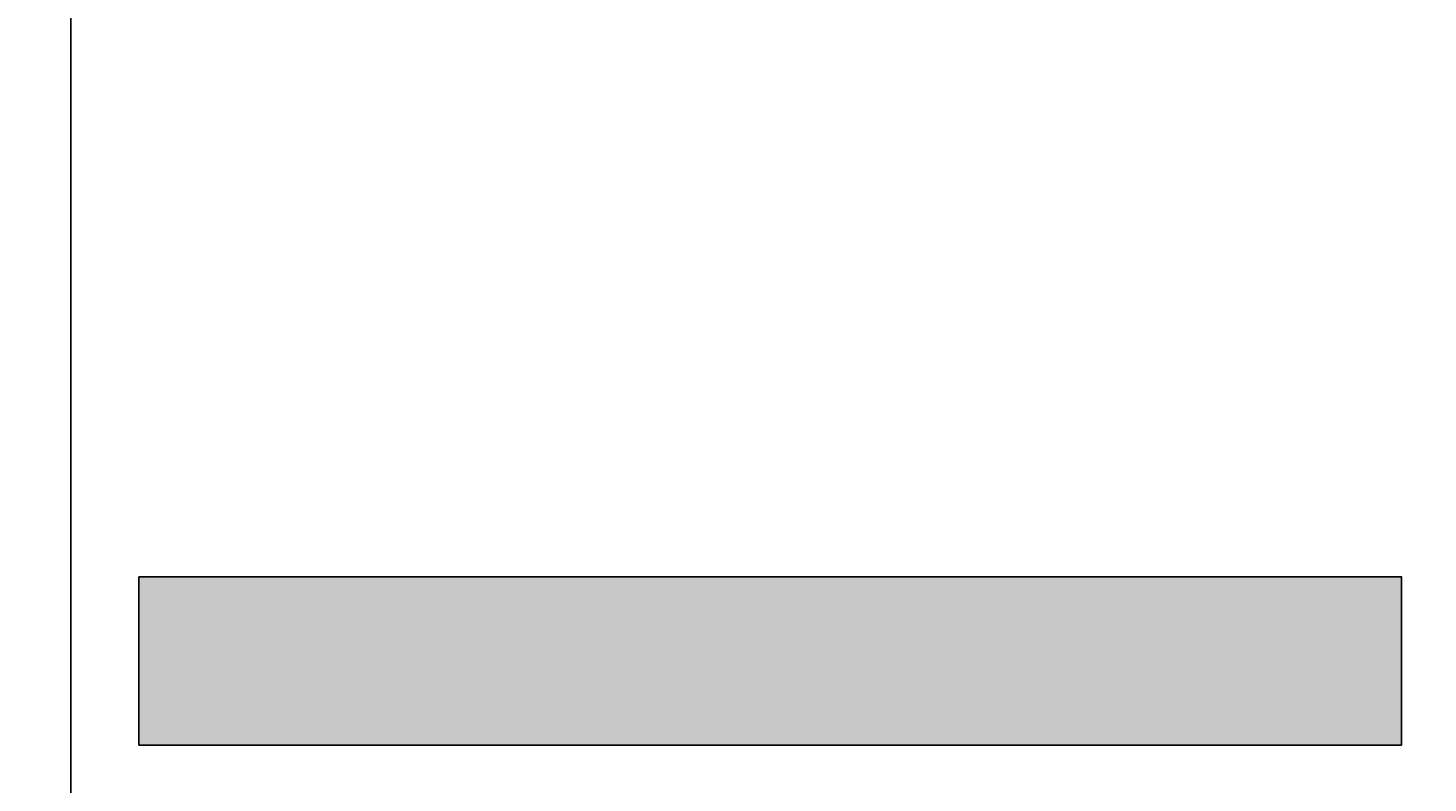
# Model space of a CAD drawing. Units: millimetres. Extents: x -11 to 280, y -4 to 208.
# Tile 3 of 55: x 28 to 61, y 36 to 54. Entities that reach past the tile are written whole.
import ezdxf

# ---------------------------------------------------------------- set-up
doc = ezdxf.new("R2010")
doc.units = ezdxf.units.MM
doc.layers.add('M-DIMS', color=2, linetype='Continuous', lineweight=18)
doc.layers.add('M-HYDR-SUCT', color=7, linetype='Continuous', lineweight=25)
doc.layers.add('M-HYDR-SUCT-PATT', color=221, linetype='Continuous', lineweight=13, true_color=0xff7fdf)
doc.styles.get("Standard").update_dxf_attribs({"font": 'arial.ttf'})
doc.dimstyles.get("Standard").update_dxf_attribs({"dimtxt": 0.18, "dimasz": 0.18, "dimexe": 0.18, "dimexo": 0.0625, "dimgap": 0.09, "dimtad": 0, "dimtih": 1, "dimtoh": 1, "dimdec": 4, "dimzin": 0, "dimdsep": 46, "dimtxsty": 'Standard', "dimcen": 0.09, "dimadec": 0, "dimazin": 0, "dimtfac": 1, "dimtdec": 4, "dimtofl": 0, "dimtmove": 0, "dimatfit": 3, "dimfxl": 1, "dimtolj": 1, "dimtzin": 0, "dimarcsym": 0})

# ---------------------------------------------------------------- blocks, each defined once
blk = doc.blocks.new('*D4')
at = {"layer": 'Defpoints', "color": 0, "transparency": 16777216}
for p in [(4.763, 84.426), (266.035, 51.733), (266.035, -3.415)]:
    blk.add_point(p, dxfattribs=at)
at = {"layer": 'M-DIMS', "color": 0, "lineweight": -2, "transparency": 16777216}
for p, q in [((4.763, 84.364), (4.763, -3.595)), ((266.035, 51.67), (266.035, -3.595)), ((4.943, -3.415), (134.934, -3.415)), ((265.855, -3.415), (135.864, -3.415))]:
    blk.add_line(p, q, dxfattribs=at)
at = {"layer": 'M-DIMS', "color": 0, "transparency": 16777216}
for points in [[(4.943, -3.385), (4.943, -3.445), (4.763, -3.415)], [(265.855, -3.385), (265.855, -3.445), (266.035, -3.415)]]:
    blk.add_solid(points, dxfattribs=at)
at = {"layer": 'M-DIMS', "color": 0, "transparency": 16777216, "insert": (135.399, -3.415), "char_height": 0.18, "attachment_point": 5}
blk.add_mtext('\\A1;261.27', dxfattribs=at)
blk = doc.blocks.new('*D5')
at = {"layer": 'Defpoints', "color": 0, "transparency": 16777216}
for p in [(24.759, 192.645), (-10.087, 11.435), (261.686, 11.435)]:
    blk.add_point(p, dxfattribs=at)
at = {"layer": 'M-DIMS', "color": 0, "lineweight": -2, "transparency": 16777216}
for p, q in [((24.696, 192.645), (-10.267, 192.645)), ((-10.087, 192.465), (-10.087, 102.222)), ((-10.087, 11.615), (-10.087, 101.858)), ((261.624, 11.435), (-10.267, 11.435))]:
    blk.add_line(p, q, dxfattribs=at)
at = {"layer": 'M-DIMS', "color": 0, "transparency": 16777216}
for points in [[(-10.117, 192.465), (-10.057, 192.465), (-10.087, 192.645)], [(-10.117, 11.615), (-10.057, 11.615), (-10.087, 11.435)]]:
    blk.add_solid(points, dxfattribs=at)
at = {"layer": 'M-DIMS', "color": 0, "transparency": 16777216, "insert": (-10.087, 102.04), "char_height": 0.18, "attachment_point": 5}
blk.add_mtext('\\A1;181.2', dxfattribs=at)
blk = doc.blocks.new('*D23')
at = {"layer": 'Defpoints', "color": 0, "transparency": 16777216}
for p in [(29.201, 153.977), (66.388, 153.977), (66.388, -3.415)]:
    blk.add_point(p, dxfattribs=at)
at = {"layer": 'M-DIMS', "color": 0, "lineweight": -2, "transparency": 16777216}
for p, q in [((29.201, 153.914), (29.201, -3.595)), ((66.388, 153.914), (66.388, -3.595)), ((29.381, -3.415), (47.331, -3.415)), ((66.208, -3.415), (48.258, -3.415))]:
    blk.add_line(p, q, dxfattribs=at)
at = {"layer": 'M-DIMS', "color": 0, "transparency": 16777216}
for points in [[(29.381, -3.385), (29.381, -3.445), (29.201, -3.415)], [(66.208, -3.385), (66.208, -3.445), (66.388, -3.415)]]:
    blk.add_solid(points, dxfattribs=at)
at = {"layer": 'M-DIMS', "color": 0, "transparency": 16777216, "insert": (47.795, -3.415), "char_height": 0.18, "attachment_point": 5}
blk.add_mtext('\\A1;37.186', dxfattribs=at)

msp = doc.modelspace()

# ---------------------------------------------------------------- hatches: boundary and pattern name
at = {"layer": 'M-HYDR-SUCT-PATT'}
h = msp.add_hatch(color=256, dxfattribs=at)
h.set_gradient(color1=(255, 127, 223), color2=(255, 127, 223), tint=1, name='INVCYLINDER')
h.paths.add_polyline_path([(91.3629, 155.4768), (91.3629, 132.4768), (58.3629, 132.4768), (58.3629, 153.9768), (54.8629, 153.9768), (54.8629, 128.9768), (94.8629, 128.9768), (94.8629, 151.9768), (205.5315, 151.9768), (205.5315, 155.4768)])
h.paths.add_polyline_path([(91.3, 114.9452, 1), (78.8273, 114.9452), (78.8273, 108.8141), (42.6453, 108.8141), (42.6453, 153.9768), (39.1453, 153.9768), (39.1453, 105.3141), (78.8273, 105.3141), (78.8273, 98.1491, 1), (91.3, 98.1491), (91.3, 105.3141), (95.5776, 105.3141), (95.5776, 108.8141), (91.3, 108.8141)])
h.paths.add_polyline_path([(228.7, 138.4081), (232.2, 138.4081), (232.2, 144.6609), (228.7, 144.6609)])
h.paths.add_polyline_path([(253.1005, 151.9768, 1), (253.1005, 155.4768), (252.6001, 155.4768), (253.5249, 153.991, -0.1401047), (253.6005, 153.7268, -0.7542249), (252.676, 153.4626), (251.4221, 155.4768), (236.9353, 155.4768), (236.9353, 151.9768)])
h.paths.add_polyline_path([(30.8182, 40.7626), (30.8182, 36.7626), (60.8182, 36.7626), (60.8182, 40.7626)])

# ---------------------------------------------------------------- linework, layer by layer
at = {"layer": 'M-HYDR-SUCT'}
msp.add_lwpolyline([(30.8182, 40.7626), (60.8182, 40.7626), (60.8182, 36.7626), (30.8182, 36.7626)], close=True, dxfattribs=at)

# ---------------------------------------------------------------- dimensions: what is measured, and where the dimension line sits
at = {"layer": 'M-DIMS'}
dim = msp.add_linear_dim(base=(-10.0865, 11.4346), p1=(24.7588, 192.645), p2=(261.6863, 11.4346), angle=90, dimstyle='Standard', override={"dimdec": 1, "dimlfac": 1, "dimrnd": 0, "dimzin": 0, "dimdsep": 46, "dimlunit": 2}, dxfattribs=at)
dim.commit()
dim.dimension.update_dxf_attribs({"geometry": '*D5', "text_midpoint": (-10.0865, 102.0398)})
for base, p1, p2, override, picture, middle in [((66.3875, -3.4154), (29.2015, 153.9768), (66.3875, 153.9768), {"dimdec": 3, "dimlfac": 1, "dimrnd": 0, "dimzin": 0, "dimdsep": 46, "dimlunit": 2}, '*D23', (47.7945, -3.4154)), ((266.0352, -3.4154), (4.7635, 84.4261), (266.0352, 51.7328), {"dimdec": 2, "dimlfac": 1, "dimrnd": 0, "dimzin": 0, "dimdsep": 46, "dimlunit": 2}, '*D4', (135.3993, -3.4154))]:
    dim = msp.add_linear_dim(base=base, p1=p1, p2=p2, dimstyle='Standard', override=override, dxfattribs=at)
    dim.commit()
    dim.dimension.update_dxf_attribs({"geometry": picture, "text_midpoint": middle})

doc.saveas('drawing.dxf')
